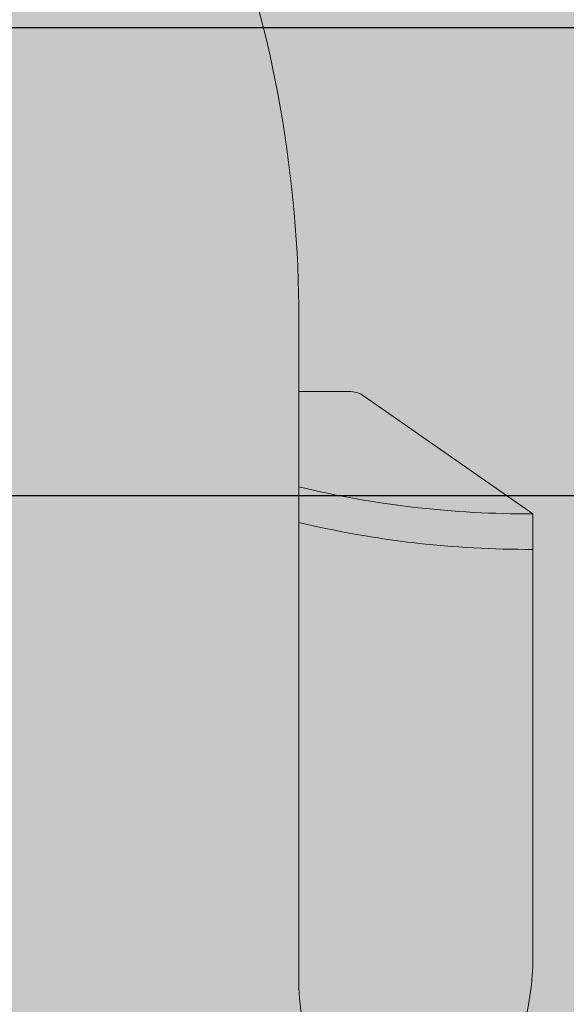
# Model space of a CAD drawing. Units: inches. Extents: x 389 to 971, y 148 to 870.
# Tile 2 of 14: x 515 to 529, y 364 to 389. Entities that reach past the tile are written whole.
import ezdxf

# ---------------------------------------------------------------- set-up
doc = ezdxf.new("R2010")
doc.units = ezdxf.units.IN
doc.header["$MEASUREMENT"] = 0
for name, color, linetype, lineweight in [('A-ANNO-DIMS', 2, 'Continuous', 18), ('C-VEHI', 8, 'Continuous', 13), ('L-GRND-BASE-PATT', 8, 'Continuous', 13)]:
    doc.layers.add(name, color=color, linetype=linetype, lineweight=lineweight)
doc.layers.add('C-VEHI-PATT', color=18, linetype='Continuous', lineweight=13, true_color=0x000000)
doc.layers.add('L-GRND-PATT', color=39, linetype='Continuous', lineweight=13, true_color=0x603913)
doc.styles.get("Standard").update_dxf_attribs({"font": 'arial.ttf'})
doc.dimstyles.get("Standard").update_dxf_attribs({"dimtxt": 8, "dimasz": 8, "dimexe": 0.18, "dimexo": 0.0625, "dimgap": 0.09, "dimtad": 0, "dimtih": 1, "dimtoh": 1, "dimdec": 0, "dimzin": 0, "dimdsep": 46, "dimlunit": 3, "dimtxsty": 'Standard', "dimcen": 0.09, "dimadec": 0, "dimazin": 0, "dimtfac": 1, "dimtdec": 0, "dimtofl": 0, "dimtmove": 0, "dimatfit": 3, "dimfxl": 1, "dimtolj": 1, "dimtzin": 0, "dimarcsym": 0})

# ---------------------------------------------------------------- blocks, each defined once
blk = doc.blocks.new('*U7')
for p, q in [((32.26591480791686, 11.62530558863241), (36.12873726252356, 17.16961494239206)), ((36.12873726252356, 17.16961494239206), (50.93891189819171, 17.16961494239206)), ((32.12291633764599, 9.505833383620029), (32.12291633764599, 11.15369945057711)), ((29.77279020470884, 9.505833383620029), (51.68362801571248, 9.505833383620029))]:
    blk.add_line(p, q)
for centre, major_axis, ratio, start_param, end_param in [((13.03653510440275, 17.00972444508943), (1.2303e-12, 27.41599049210566), 0.8423038695439277, 4.435146050259648, 4.718221029521873), ((14.20086229321332, 17.00972444508943), (1.2303e-12, 27.41599049210566), 0.8423038695439277, 4.435146050259648, 4.718221029521873), ((50.7902773840875, 13.33772416300607), (6.340077547122382, -0.356608581037027), 0.6038335755719145, -1.39555193967809, 1.581314658479915), ((32.74615637525823, 11.15369945057713), (1.313e-13, 0.7399230374541176), 0.8423038695439091, 0.8797135699495516, 1.570796326795045), ((29.77279020470884, -46.66302566589627), (5.12e-14, 56.16885904951626), 0.842303869543976, 7e-16, 0.5903187773915901)]:
    blk.add_ellipse(centre, major_axis=major_axis, ratio=ratio, start_param=start_param, end_param=end_param)
blk = doc.blocks.new('*D53')
at = {"layer": 'A-ANNO-DIMS', "color": 0, "lineweight": -2, "transparency": 16777216}
for p, q in [((397.8910240000004, 396.9189020000002), (397.8910240000004, 404.9189020000001)), ((690.1535240000002, 388.9189020000003), (397.7110240000004, 388.9189020000002)), ((690.1535240000002, 376.9189020000001), (397.7110240000005, 376.9189020000001)), ((397.8910240000005, 368.9189020000001), (397.8910240000005, 360.918902))]:
    blk.add_line(p, q, dxfattribs=at)
at = {"layer": 'A-ANNO-DIMS', "color": 0, "transparency": 16777216}
for points in [[(396.5576906666671, 396.9189020000002), (399.2243573333337, 396.9189020000002), (397.8910240000004, 388.9189020000002)], [(396.5576906666671, 368.9189020000001), (399.2243573333338, 368.9189020000001), (397.8910240000005, 376.9189020000001)]]:
    blk.add_solid(points, dxfattribs=at)
at = {"layer": 'Defpoints', "color": 0, "transparency": 16777216}
for p in [(397.8910240000004, 388.9189020000002), (690.2160240000001, 388.9189020000003), (690.2160240000001, 376.9189020000001)]:
    blk.add_point(p, dxfattribs=at)
at = {"layer": 'A-ANNO-DIMS', "color": 0, "transparency": 16777216, "insert": (397.8910240000004, 382.9189019999999), "char_height": 8, "attachment_point": 5}
blk.add_mtext('\\A1;12', dxfattribs=at)

msp = doc.modelspace()

# ---------------------------------------------------------------- hatches: boundary and pattern name
at = {"layer": 'C-VEHI-PATT'}
h = msp.add_hatch(color=256, dxfattribs=at)
h.dxf.hatch_style = 1
edge = h.paths.add_edge_path()
edge.add_ellipse((550.9021553826709, 381.4331108862803), major_axis=(-43.99405423656321, 1.9369e-12), ratio=0.8423038695439613, start_angle=-29.43856959797762, end_angle=1.8189894035458565e-12, ccw=False)
edge.add_line((514.3535105156315, 402.059641051582), (514.3535105156315, 404.7525403567118))
edge.add_ellipse((514.3535105156316, 404.2643898676136), major_axis=(0.5795420236673633, 2e-16), ratio=0.8423038695437671, start_angle=90.00000000001334, end_angle=127.9331304598466)
edge.add_line((514.0354569934393, 404.6724605914631), (509.5535496243029, 402.1940957519602))
edge.add_ellipse((473.3138688667988, 564.9222417143382), major_axis=(196.5636751472093, 8.4793e-12), ratio=0.8423038695439335, start_angle=-80.7434339928015, end_angle=-77.44506735586577, ccw=False)
edge.add_ellipse((535.9119176052684, 201.7546502845751), major_axis=(239.1273775699096, 1.008988e-10), ratio=0.842303869543627, start_angle=100.2095389971183, end_angle=102.4446272934191)
edge.add_ellipse((979.5722266908713, 375.4013592680145), major_axis=(-488.2195497741742, 7.7268e-12), ratio=0.842303869543895, start_angle=-2.863714607837472, end_angle=2.198540565955285)
edge.add_ellipse((510.1338164488812, 299.4839331720496), major_axis=(70.3178640738586, 3.814e-12), ratio=0.8423038695439212, start_angle=94.08241069114638, end_angle=107.71995322274631, ccw=False)
edge.add_line((505.914122382133, 358.6062023341113), (522.79289864913, 358.606202334111))
edge.add_ellipse((518.5732045823792, 299.4839331720493), major_axis=(-70.31786407385354, 1.4408e-12), ratio=0.8423038695439844, start_angle=252.2800467772501, end_angle=265.91758930884987, ccw=False)
edge.add_ellipse((49.13479434038987, 375.4013592680261), major_axis=(-488.2195497741754, 2.5232e-12), ratio=0.8423038695439587, start_angle=177.8014594340444, end_angle=182.8637146078372)
edge.add_ellipse((492.795103425985, 201.7546502845724), major_axis=(239.12737756976, 4.82267e-11), ratio=0.8423038695441539, start_angle=77.5553727065425, end_angle=79.79046100284327)
edge.add_ellipse((555.3931521644682, 564.9222417143374), major_axis=(-196.5636751472384, 3.62381e-11), ratio=0.8423038695438114, start_angle=77.4450673558726, end_angle=80.74343399280832, ccw=False)
edge.add_line((519.1534714069603, 402.19409575196), (514.671564037824, 404.6724605914631))
edge.add_ellipse((514.3535105156316, 404.2643898676136), major_axis=(0.5795420236673633, 2e-16), ratio=0.8423038695437671, start_angle=52.06686954015338, end_angle=90.00000000001334)
edge.add_line((514.3535105156315, 404.7525403567118), (514.3535105156315, 402.0596410515821))
edge.add_ellipse((477.8048656485917, 381.4331108862812), major_axis=(-43.99405423656326, 6.67e-13), ratio=0.8423038695439753, start_angle=180.0000000000002, end_angle=209.4385695979796, ccw=False)
edge.add_line((521.7989198851549, 381.4331108862806), (521.7989198851549, 379.5923831537828))
edge.add_line((521.7989198851549, 379.5923831537828), (523.2258361412675, 379.5923831537828))
edge.add_ellipse((523.0896049791924, 379.1042326646847), major_axis=(0.5795420236669786, 3.601e-13), ratio=0.8423038695443263, start_angle=45.519789117397124, end_angle=89.99999999996442, ccw=False)
edge.add_line((523.4589887688404, 379.4803801228631), (527.8015488731598, 376.4548385069232))
edge.add_line((527.8015488731598, 376.4548385069232), (527.8015488731597, 364.8548231745798))
edge.add_ellipse((524.8002343791572, 364.9712406163019), major_axis=(0.279312372030448, 4.96584264291768), ratio=0.6038335755719146, start_angle=106.34259195429831, end_angle=270.9979857249735, ccw=False)
edge.add_line((521.7989198851548, 364.2715269884119), (521.7989198851549, 381.4331108862806))
edge.add_ellipse((477.8048656485917, 381.4331108862812), major_axis=(-43.99405423656326, 6.67e-13), ratio=0.8423038695439753, start_angle=180.0000000000001, end_angle=209.4385695979795)
edge.add_ellipse((550.9021553826709, 381.4331108862803), major_axis=(-43.99405423656321, 1.9369e-12), ratio=0.8423038695439613, start_angle=-29.43856959797755, end_angle=1.8539e-12)
edge.add_line((506.9081011461076, 381.43311088628), (506.9081011461074, 364.2715269884121))
edge.add_ellipse((503.9067866521049, 364.9712406163021), major_axis=(-0.2793123720310282, 4.965842642917721), ratio=0.6038335755718928, start_angle=89.00201427501901, end_angle=253.6574080456941, ccw=False)
edge.add_line((500.9054721581025, 364.8548231745812), (500.9054721581025, 376.4548385069235))
edge.add_line((500.9054721581025, 376.4548385069235), (505.3530060491612, 379.5535172937331))
edge.add_ellipse((505.61741605207, 379.1042326646849), major_axis=(-0.5795420236672051, 1.236e-13), ratio=0.842303869543997, start_angle=-89.99999999998778, end_angle=-45.51978911742469, ccw=False)
edge.add_line((505.61741605207, 379.5923831537831), (506.9081011461076, 379.5923831537831))
edge.add_line((506.9081011461076, 379.5923831537831), (506.9081011461076, 381.43311088628))
h = msp.add_hatch(color=256, dxfattribs=at)
h.dxf.hatch_style = 1
edge = h.paths.add_edge_path()
edge.add_ellipse((492.795103425985, 201.7546502845724), major_axis=(239.12737756976, 4.82267e-11), ratio=0.8423038695441539, start_angle=77.5553727065425, end_angle=79.79046100284327)
edge.add_ellipse((555.3931521644682, 564.9222417143374), major_axis=(-196.5636751472384, 3.62381e-11), ratio=0.8423038695438114, start_angle=77.4450673558726, end_angle=80.74343399280832, ccw=False)
edge.add_line((519.1534714069603, 402.19409575196), (519.1534714069603, 394.0892586662818))
edge.add_ellipse((477.8048656485917, 381.4331108862812), major_axis=(-43.99405423656326, 6.67e-13), ratio=0.8423038695439753, start_angle=180.0000000000002, end_angle=197.0185128172791, ccw=False)
edge.add_line((521.7989198851549, 381.4331108862806), (521.7989198851549, 379.5923831537828))
edge.add_line((521.7989198851549, 379.5923831537828), (523.1794038652976, 379.5923831537828))
edge.add_ellipse((523.0896049791924, 379.1042326646847), major_axis=(0.5795420236669786, 3.601e-13), ratio=0.8423038695443263, start_angle=45.519789117397124, end_angle=89.99999999996442, ccw=False)
edge.add_line((523.4589887688405, 379.480380122863), (527.8015488731598, 376.4548385069232))
edge.add_line((527.8015488731598, 376.4548385069232), (527.8015488731597, 364.8548231745798))
edge.add_ellipse((524.8002343791572, 364.9712406163019), major_axis=(0.279312372030448, 4.96584264291768), ratio=0.6038335755719146, start_angle=106.34259195429831, end_angle=270.9979857249735, ccw=False)
edge.add_line((521.7989198851548, 364.2715269884119), (521.7989198851549, 381.4331108862806))
edge.add_ellipse((477.8048656485917, 381.4331108862812), major_axis=(-43.99405423656326, 6.67e-13), ratio=0.8423038695439753, start_angle=180.0000000000001, end_angle=197.018512817279)
edge.add_line((519.1534714069603, 394.0892586662818), (519.1534714069603, 358.6062023341111))
edge.add_line((519.1534714069603, 358.6062023341111), (522.79289864913, 358.606202334111))
edge.add_ellipse((518.5732045823792, 299.4839331720493), major_axis=(-70.31786407385354, 1.4408e-12), ratio=0.8423038695439844, start_angle=252.2800467772501, end_angle=265.91758930884987, ccw=False)
edge.add_ellipse((49.13479434038987, 375.4013592680261), major_axis=(-488.2195497741754, 2.5232e-12), ratio=0.8423038695439587, start_angle=177.8014594340444, end_angle=182.8637146078372)
h = msp.add_hatch(color=256, dxfattribs=at)
h.dxf.hatch_style = 1
edge = h.paths.add_edge_path(flags=16)
edge.add_ellipse((3386.011413077446, 329.726312794031), major_axis=(-2896.629999631248, 1.069454e-10), ratio=0.8423038695494893, start_angle=-0.1208973690315247, end_angle=0.3640763488915013, ccw=False)
edge.add_line((489.3905023836935, 335.8383575186984), (486.2179253655185, 346.1978202249628))
edge.add_ellipse((8782.002602781096, 354.247254279773), major_axis=(-8295.790181758603, 9.87839e-10), ratio=0.8423038695486498, start_angle=0.0555943135052214, end_angle=0.3777641939157137)
edge.add_line((486.4665645878948, 299.5520931219791), (489.4638383140943, 311.3204429697198))
edge = h.paths.add_edge_path(flags=16)
edge.add_ellipse((512.1608573463288, 287.5825181681774), major_axis=(62.33048198263887, 2.0798e-12), ratio=0.8423038695439498, start_angle=94.8700695971331, end_angle=112.791914877584)
edge.add_line((491.3642517254777, 337.0752369161335), (489.6529508739416, 349.9015767089268))
edge.add_ellipse((510.1338164488795, 298.7862183048575), major_axis=(64.04807894948699, 3.9006e-12), ratio=0.8423038695439252, start_angle=94.27742096304979, end_angle=111.83495379670401, ccw=False)
edge.add_line((506.1068129054811, 352.6274231954524), (522.600208125781, 352.6274231954521))
edge.add_ellipse((518.5732045823798, 298.7862183048586), major_axis=(64.04807894948067, 3.24e-14), ratio=0.8423038695439885, start_angle=68.16504620328948, end_angle=85.72257903694378, ccw=False)
edge.add_line((539.05407015732, 349.9015767089259), (537.3427693057835, 337.0752369161327))
edge.add_ellipse((516.5461636849332, 287.5825181681899), major_axis=(62.33048198262021, 1.5954e-12), ratio=0.8423038695439995, start_angle=67.20808512240782, end_angle=85.12993040286212)
edge.add_line((521.0080028322477, 339.9490379899644), (507.6990181990146, 339.9490379899646))
edge = h.paths.add_edge_path(flags=16)
edge.add_ellipse((514.3535105156315, 391.3730654902235), major_axis=(-115.1512533244504, 1.8736e-12), ratio=0.8423038695439684, start_angle=76.4018653097696, end_angle=103.5981346902308)
edge.add_line((537.3427693057832, 296.3333211885938), (537.342769305783, 281.5897392316151))
edge.add_ellipse((514.3535105156313, 376.6294835332447), major_axis=(-115.1512533244486, 9.02e-13), ratio=0.8423038695439828, start_angle=76.40186530976922, end_angle=103.59813469023032, ccw=False)
edge.add_line((491.3642517254773, 281.5897392316156), (491.3642517254774, 296.3333211885945))
edge = h.paths.add_edge_path()
edge.add_ellipse((8782.002602781105, 354.2472542798386), major_axis=(-8296.949265805946, 5.39345e-11), ratio=0.8423038695428886, start_angle=0.3838667787920247, end_angle=0.5282714718170651)
edge.add_ellipse((8782.002602781105, 354.2472542798386), major_axis=(-8296.949265805946, 5.39345e-11), ratio=0.8423038695428886, start_angle=0.5282714718170651, end_angle=0.6465540970606384)
edge.add_ellipse((488.1158467995968, 260.6509346628684), major_axis=(2.318168094668909, 7.48e-14), ratio=0.8423038695439647, start_angle=180.6465540970884, end_angle=269.9999999999081)
edge.add_line((488.115846799593, 258.6983327064755), (491.3642517254771, 258.6983327064753))
edge.add_line((491.3642517254771, 258.6983327064753), (491.3642517254771, 274.201106836649))
edge.add_ellipse((493.6824198201462, 273.9438556676354), major_axis=(-2.318168094668919, 1.896e-13), ratio=0.8423038695439611, start_angle=-89.99999999999523, end_angle=4.718003765447065e-12, ccw=False)
edge.add_line((493.6824198201462, 275.8964576240284), (535.3300149439905, 275.8964576240277))
edge.add_ellipse((535.024601211114, 273.9438556676347), major_axis=(2.318168094668976, 2.946e-13), ratio=0.8423038695439647, start_angle=-7.275957614183426e-12, end_angle=89.99999999998943, ccw=False)
edge.add_line((537.342769305783, 273.9438556676347), (537.3427693057827, 258.698332706474))
edge.add_line((537.3427693057827, 258.698332706474), (540.591174231666, 258.6983327064739))
edge.add_ellipse((540.5911742316634, 260.6509346628669), major_axis=(-2.318168094668839, 2.143e-13), ratio=0.8423038695440144, start_angle=90.00000000008203, end_angle=179.3534459029346)
edge.add_ellipse((-7753.295581726658, 354.2472542799028), major_axis=(-8296.949265782761, 2.068448e-10), ratio=0.8423038695442414, start_angle=179.3534459029388, end_angle=179.3813568036815)
edge.add_ellipse((-7753.295581726658, 354.2472542799028), major_axis=(-8296.949265782761, 2.068448e-10), ratio=0.8423038695442414, start_angle=179.3813568036815, end_angle=179.4717285281828)
edge.add_ellipse((-7753.295581726658, 354.2472542799028), major_axis=(-8296.949265782761, 2.068448e-10), ratio=0.8423038695442414, start_angle=179.4717285281828, end_angle=179.6161332212082)
edge.add_ellipse((-7753.295581726658, 354.2472542799028), major_axis=(-8296.949265782761, 2.068448e-10), ratio=0.8423038695442414, start_angle=179.6161332212082, end_angle=180.090229088595)
edge.add_ellipse((-7753.295581726658, 354.2472542799028), major_axis=(-8296.949265782761, 2.068448e-10), ratio=0.8423038695442414, start_angle=180.090229088595, end_angle=180.134986576859)
edge.add_ellipse((129.8867725257751, 372.4897205359271), major_axis=(-413.7373561031673, 2.44623e-11), ratio=0.8423038695441432, start_angle=180.1806905311865, end_angle=182.1799503136479)
edge.add_ellipse((129.8867725257751, 372.4897205359271), major_axis=(-413.7373561031673, 2.44623e-11), ratio=0.8423038695441432, start_angle=182.1799503136479, end_angle=183.6504275857017)
edge.add_ellipse((492.7951034259847, 196.3854951855023), major_axis=(245.3971626940514, 1.422861e-10), ratio=0.8423038695444116, start_angle=76.21947101046817, end_angle=77.87403444768196)
edge.add_ellipse((49.13479434038987, 375.4013592680261), major_axis=(-488.2195497741754, 2.5232e-12), ratio=0.8423038695439587, start_angle=177.8014594340445, end_angle=182.8637146078372, ccw=False)
edge.add_ellipse((518.5732045823792, 299.4839331720493), major_axis=(-70.31786407385354, 1.4408e-12), ratio=0.8423038695439844, start_angle=252.2800467772501, end_angle=265.9175893088498)
edge.add_line((522.79289864913, 358.606202334111), (505.9141223821329, 358.6062023341113))
edge.add_ellipse((510.1338164488812, 299.4839331720496), major_axis=(70.3178640738586, 3.814e-12), ratio=0.8423038695439212, start_angle=94.08241069114636, end_angle=107.7199532227462)
edge.add_ellipse((979.5722266908713, 375.4013592680145), major_axis=(-488.2195497741742, 7.7268e-12), ratio=0.842303869543895, start_angle=-2.863714607837494, end_angle=2.198540565955284, ccw=False)
edge.add_ellipse((535.9119176052733, 196.3854951855018), major_axis=(-245.3971626940985, 1.013648e-10), ratio=0.8423038695442548, start_angle=-77.87403444769295, end_angle=-76.2194710104792)
edge.add_ellipse((898.8202485054873, 372.489720535918), major_axis=(413.7373561031672, 1.26113e-11), ratio=0.8423038695441164, start_angle=176.3495724142985, end_angle=177.8200496863523)
edge.add_ellipse((898.8202485054873, 372.489720535918), major_axis=(413.7373561031672, 1.26113e-11), ratio=0.8423038695441164, start_angle=177.8200496863523, end_angle=179.8643876095591)
edge.add_ellipse((8782.002602781105, 354.2472542798386), major_axis=(-8296.949265805946, 5.39345e-11), ratio=0.8423038695428886, start_angle=-0.1349865768573029, end_angle=-0.090229088593484)
edge.add_ellipse((8782.002602781105, 354.2472542798386), major_axis=(-8296.949265805946, 5.39345e-11), ratio=0.8423038695428886, start_angle=-0.090229088593484, end_angle=0.3838667787920247)
edge = h.paths.add_edge_path(flags=16)
edge.add_ellipse((-2357.304392046186, 329.7263127941099), major_axis=(2896.629999631251, 5.35614e-11), ratio=0.8423038695445265, start_angle=-0.3640763488920631, end_angle=0.1208973690309369)
edge.add_line((539.3165186475693, 335.8383575187012), (542.4890956657468, 346.1978202249727))
edge.add_ellipse((-7753.295581749842, 354.2472542800017), major_axis=(8295.790181758617, 3.2664368e-09), ratio=0.8423038695525207, start_angle=-0.37776419393310334, end_angle=-0.055594313522590255, ccw=False)
edge.add_line((542.240456443367, 299.5520931219743), (539.2431827171666, 311.3204429697195))
h = msp.add_hatch(color=256, dxfattribs=at)
h.dxf.hatch_style = 1
edge = h.paths.add_edge_path()
edge.add_ellipse((523.0896049791924, 379.1042326646847), major_axis=(0.5795420236669786, 3.601e-13), ratio=0.8423038695443263, start_angle=45.51978911739708, end_angle=89.99999999996442)
edge.add_line((523.0896049791935, 379.5923831537828), (521.7989198851549, 379.5923831537828))
edge.add_line((521.7989198851549, 379.5923831537828), (521.7989198851549, 377.1452135063881))
edge.add_ellipse((527.6763152236028, 394.5417217261543), major_axis=(-21.47347468097256, 2.8383e-12), ratio=0.8423038695438576, start_angle=71.33250450740293, end_angle=90.39670985998444)
edge.add_line((527.8015488731598, 376.4548385069232), (523.4589887688408, 379.4803801228628))
h = msp.add_hatch(color=256, dxfattribs=at)
h.dxf.hatch_style = 1
edge = h.paths.add_edge_path()
edge.add_ellipse((523.0896049791924, 379.1042326646847), major_axis=(0.5795420236669786, 3.601e-13), ratio=0.8423038695443263, start_angle=45.51978911739708, end_angle=89.99999999996442)
edge.add_line((523.0896049791935, 379.5923831537828), (521.7989198851549, 379.5923831537828))
edge.add_line((521.7989198851549, 379.5923831537828), (521.7989198851549, 377.1452135063881))
edge.add_ellipse((527.6763152236028, 394.5417217261543), major_axis=(-21.47347468097256, 2.8383e-12), ratio=0.8423038695438576, start_angle=71.33250450740293, end_angle=90.39670985998444)
edge.add_line((527.8015488731598, 376.4548385069232), (523.4589887688408, 379.4803801228628))
h = msp.add_hatch(color=256, dxfattribs=at)
h.dxf.hatch_style = 1
edge = h.paths.add_edge_path()
edge.add_ellipse((523.0896049791924, 379.1042326646847), major_axis=(0.5795420236669786, 3.601e-13), ratio=0.8423038695443263, start_angle=45.51978911739708, end_angle=89.99999999996442)
edge.add_line((523.0896049791935, 379.5923831537828), (521.7989198851549, 379.5923831537828))
edge.add_line((521.7989198851549, 379.5923831537828), (521.7989198851549, 377.1452135063881))
edge.add_ellipse((527.6763152236028, 394.5417217261543), major_axis=(-21.47347468097256, 2.8383e-12), ratio=0.8423038695438576, start_angle=71.33250450740293, end_angle=90.39670985998444)
edge.add_line((527.8015488731598, 376.4548385069232), (523.4589887688408, 379.4803801228628))
h = msp.add_hatch(color=256, dxfattribs=at)
h.dxf.hatch_style = 1
edge = h.paths.add_edge_path()
edge.add_ellipse((527.6763152236028, 394.5417217261543), major_axis=(-21.47347468097256, 2.8383e-12), ratio=0.8423038695438576, start_angle=71.33250450740297, end_angle=90.39670985998453, ccw=False)
edge.add_line((521.7989198851549, 377.1452135063881), (521.7989198851549, 376.2332584772058))
edge.add_ellipse((527.6763152236027, 393.629766696972), major_axis=(-21.47347468097092, 1.1981e-12), ratio=0.8423038695439196, start_angle=71.33250450739882, end_angle=90.3967098599804)
edge.add_line((527.8015488731598, 375.5428834777409), (527.8015488731598, 376.4548385069232))
h = msp.add_hatch(color=256, dxfattribs=at)
h.dxf.hatch_style = 1
edge = h.paths.add_edge_path()
edge.add_ellipse((527.6763152236027, 393.629766696972), major_axis=(-21.47347468097092, 1.1981e-12), ratio=0.8423038695439196, start_angle=71.33250450739882, end_angle=90.39670985998049, ccw=False)
edge.add_line((521.7989198851549, 376.2332584772058), (521.7989198851548, 364.2715269884119))
edge.add_ellipse((524.8002343791572, 364.9712406163019), major_axis=(0.279312372030448, 4.96584264291768), ratio=0.6038335755719146, start_angle=106.3425919542983, end_angle=270.9979857249735)
edge.add_line((527.8015488731597, 364.8548231745798), (527.8015488731598, 375.5428834777409))
h = msp.add_hatch(color=256, dxfattribs=at)
h.dxf.hatch_style = 1
edge = h.paths.add_edge_path()
edge.add_ellipse((527.6763152236027, 393.629766696972), major_axis=(-21.47347468097092, 1.1981e-12), ratio=0.8423038695439196, start_angle=71.33250450739882, end_angle=90.39670985998049, ccw=False)
edge.add_line((521.7989198851549, 376.2332584772058), (521.7989198851548, 364.2715269884119))
edge.add_ellipse((524.8002343791572, 364.9712406163019), major_axis=(0.279312372030448, 4.96584264291768), ratio=0.6038335755719146, start_angle=106.3425919542983, end_angle=270.9979857249735)
edge.add_line((527.8015488731597, 364.8548231745798), (527.8015488731598, 375.5428834777409))
at = {"layer": 'L-GRND-BASE-PATT'}
h = msp.add_hatch(color=256, dxfattribs=at)
h.dxf.hatch_style = 1
edge = h.paths.add_edge_path(flags=16)
edge.add_ellipse((8782.002602781105, 354.2472542798386), major_axis=(-8296.949265805946, 5.39345e-11), ratio=0.8423038695428886, start_angle=-0.0902290885933894, end_angle=0.3838667787920258, ccw=False)
edge.add_ellipse((485.0533369751568, 368.2895347624687), major_axis=(-1.159084047334488, 1.838e-13), ratio=0.8423038695439892, start_angle=9.094947017729282e-12, end_angle=90.00000000000898, ccw=False)
edge.add_line((483.8942529278224, 368.2895347624687), (483.8942529278225, 387.6039063360424))
edge.add_ellipse((485.0533369751571, 387.2465553762829), major_axis=(1.159084047334488, 1.838e-13), ratio=0.8423038695439892, start_angle=89.99999999999102, end_angle=179.9999999999909, ccw=False)
edge.add_line((485.0533369751572, 388.2228563544795), (485.5047440247956, 388.2228563544795))
edge.add_ellipse((898.8202485054873, 372.489720535918), major_axis=(413.7373561031672, 1.26113e-11), ratio=0.8423038695441164, start_angle=176.3495724142986, end_angle=177.8200496863524, ccw=False)
edge.add_ellipse((535.9119176052733, 196.3854951855018), major_axis=(-245.3971626940985, 1.013648e-10), ratio=0.8423038695442548, start_angle=-77.87403444769302, end_angle=-76.2194710104792, ccw=False)
edge.add_ellipse((535.9119176052684, 201.7546502845751), major_axis=(239.1273775699096, 1.008988e-10), ratio=0.842303869543627, start_angle=100.20953899711827, end_angle=102.44462729341922, ccw=False)
edge.add_ellipse((473.3138688667988, 564.9222417143382), major_axis=(196.5636751472093, 8.4793e-12), ratio=0.8423038695439335, start_angle=-80.74343399280163, end_angle=-77.44506735586587)
edge.add_line((509.5535496243029, 402.1940957519602), (514.3535105156315, 404.8483349684994))
edge.add_line((514.3535105156315, 404.8483349684994), (514.3535105156315, 404.7971763262221))
edge.add_ellipse((514.3535105156316, 404.2643898676136), major_axis=(0.5795420236673633, 2e-16), ratio=0.8423038695437671, start_angle=52.06686954015339, end_angle=90.00000000001342, ccw=False)
edge.add_line((514.671564037824, 404.672460591463), (519.1534714069603, 402.19409575196))
edge.add_ellipse((555.3931521644682, 564.9222417143374), major_axis=(-196.5636751472384, 3.62381e-11), ratio=0.8423038695438114, start_angle=77.44506735587258, end_angle=80.74343399280833)
edge.add_ellipse((492.795103425985, 201.7546502845724), major_axis=(239.12737756976, 4.82267e-11), ratio=0.8423038695441539, start_angle=77.55537270654253, end_angle=79.7904610028433, ccw=False)
edge.add_ellipse((492.7951034259847, 196.3854951855023), major_axis=(245.3971626940514, 1.422861e-10), ratio=0.8423038695444116, start_angle=76.21947101046823, end_angle=77.87403444768199, ccw=False)
edge.add_ellipse((129.8867725257751, 372.4897205359271), major_axis=(-413.7373561031673, 2.44623e-11), ratio=0.8423038695441432, start_angle=182.179950313648, end_angle=183.6504275857018, ccw=False)
edge.add_line((543.2022770064673, 388.2228563544788), (544.0779382625514, 388.2228563544787))
edge.add_ellipse((543.6536840561057, 387.2465553762822), major_axis=(-1.159084047334545, 1.527e-13), ratio=0.8423038695438989, start_angle=180.0000000000075, end_angle=270.00000000000756, ccw=False)
edge.add_line((544.8127681034401, 387.2465553762826), (544.8127681034399, 367.9321838027083))
edge.add_ellipse((543.6536840561054, 368.2895347624679), major_axis=(1.159084047334544, 7.24e-14), ratio=0.8423038695439478, start_angle=269.9999999999964, end_angle=359.9999999999964, ccw=False)
edge.add_ellipse((-7753.295581726658, 354.2472542799028), major_axis=(-8296.949265782761, 2.068448e-10), ratio=0.8423038695442414, start_angle=179.6161332212083, end_angle=180.0902290885951, ccw=False)
edge.add_line((543.3912265319653, 298.6607849184036), (544.0779382625504, 298.6607849184036))
edge.add_ellipse((543.6536840561046, 297.6844839402071), major_axis=(1.159084047334431, 1.769e-13), ratio=0.8423038695439814, start_angle=-1.1482370609883219e-11, end_angle=89.99999999999119, ccw=False)
edge.add_line((544.8127681034391, 297.684483940207), (544.8127681034387, 278.3701123666333))
edge.add_ellipse((543.6536840561043, 278.727463326393), major_axis=(-1.159084047334431, 2.574e-13), ratio=0.8423038695440306, start_angle=90.00000000001268, end_angle=180.0000000000099, ccw=False)
edge.add_line((543.6536840561045, 277.7511623481965), (543.1566278692261, 277.7511623481965))
edge.add_ellipse((-7753.295581726658, 354.2472542799028), major_axis=(-8296.949265782761, 2.068448e-10), ratio=0.8423038695442414, start_angle=179.3813568036816, end_angle=179.4717285281829, ccw=False)
edge.add_ellipse((542.4236240941387, 263.2762864208561), major_axis=(-1.738626071001761, 2.132e-13), ratio=0.8423038695439151, start_angle=179.3717627838137, end_angle=248.464756601011, ccw=False)
edge.add_ellipse((-7753.875123750511, 354.2472542780016), major_axis=(-8298.740341433751, 2.4782644722e-06), ratio=0.8423038662721074, start_angle=179.3534459200609, end_angle=179.3717628008941, ccw=False)
edge.add_ellipse((540.0116322079951, 260.6509346628677), major_axis=(-4.109243751168186, 2.384e-13), ratio=0.842303869543976, start_angle=90.0000000000635, end_angle=179.3534459029233, ccw=False)
edge.add_line((540.0116322079991, 257.1897027503593), (488.6953888232593, 257.1897027503609))
edge.add_ellipse((488.6953888232669, 260.6509346628715), major_axis=(4.10924375117072, 1.262e-13), ratio=0.8423038695439824, start_angle=180.6465540970565, end_angle=269.9999999998589, ccw=False)
edge.add_ellipse((8782.582144816053, 354.2472542821698), major_axis=(-8298.740341477976, 1.8591886369e-06), ratio=0.8423038720186145, start_angle=0.6282372290784792, end_angle=0.6465541099116194, ccw=False)
edge.add_ellipse((486.2833969371199, 263.2762864208594), major_axis=(-1.738626071002378, 2.7e-13), ratio=0.8423038695439394, start_angle=-68.46475649596817, end_angle=0.6282372161796275, ccw=False)
edge.add_ellipse((8782.002602781105, 354.2472542798386), major_axis=(-8296.949265805946, 5.39345e-11), ratio=0.8423038695428886, start_angle=0.5282714718171064, end_angle=0.6465540970606867, ccw=False)
edge.add_line((485.5503931620382, 277.7511623481972), (484.6290827687102, 277.7511623481972))
edge.add_ellipse((485.0533369751559, 278.7274633263938), major_axis=(-1.159084047334545, 3.11e-13), ratio=0.8423038695439968, start_angle=1.5404566511278972e-11, end_angle=90.000000000012, ccw=False)
edge.add_line((483.8942529278214, 278.7274633263938), (483.8942529278216, 298.0418348999672))
edge.add_ellipse((485.053336975156, 297.6844839402078), major_axis=(1.159084047334488, 1.025e-13), ratio=0.8423038695440382, start_angle=89.99999999999488, end_angle=179.9999999999949, ccw=False)
edge = h.paths.add_edge_path(flags=0)
edge.add_ellipse((8782.002602781096, 354.247254279773), major_axis=(-8295.790181758603, 9.87839e-10), ratio=0.8423038695486498, start_angle=0.05559431350519617, end_angle=0.37776419391582294, ccw=False)
edge.add_line((486.2179253655185, 346.1978202249628), (489.3905023836935, 335.8383575186984))
edge.add_ellipse((3386.011413077446, 329.726312794031), major_axis=(-2896.629999631248, 1.069454e-10), ratio=0.8423038695494893, start_angle=-0.1208973690315206, end_angle=0.3640763488915184)
edge.add_line((489.4638383140943, 311.3204429697198), (486.4665645878948, 299.5520931219791))
edge = h.paths.add_edge_path(flags=0)
edge.add_ellipse((514.3535105156315, 391.3730654902235), major_axis=(-115.1512533244504, 1.8736e-12), ratio=0.8423038695439684, start_angle=76.4018653097696, end_angle=103.5981346902308)
edge.add_line((537.3427693057832, 296.3333211885938), (537.342769305783, 281.5897392316151))
edge.add_ellipse((514.3535105156313, 376.6294835332447), major_axis=(-115.1512533244486, 9.02e-13), ratio=0.8423038695439828, start_angle=76.40186530976922, end_angle=103.59813469023032, ccw=False)
edge.add_line((491.3642517254773, 281.5897392316156), (491.3642517254774, 296.3333211885945))
edge = h.paths.add_edge_path(flags=0)
edge.add_line((491.3642517254777, 337.0752369161334), (489.6529508739416, 349.9015767089268))
edge.add_ellipse((510.1338164488795, 298.7862183048575), major_axis=(64.04807894948699, 3.9006e-12), ratio=0.8423038695439252, start_angle=94.27742096304979, end_angle=111.83495379670401, ccw=False)
edge.add_line((506.106812905481, 352.6274231954524), (522.600208125781, 352.6274231954521))
edge.add_ellipse((518.5732045823798, 298.7862183048586), major_axis=(64.04807894948067, 3.24e-14), ratio=0.8423038695439885, start_angle=68.16504620328948, end_angle=85.72257903694378, ccw=False)
edge.add_line((539.05407015732, 349.9015767089259), (537.3427693057835, 337.0752369161327))
edge.add_ellipse((516.5461636849332, 287.5825181681899), major_axis=(62.33048198262021, 1.5954e-12), ratio=0.8423038695439995, start_angle=67.20808512240782, end_angle=85.12993040286212)
edge.add_line((521.0080028322477, 339.9490379899644), (507.6990181990146, 339.9490379899646))
edge.add_ellipse((512.1608573463288, 287.5825181681774), major_axis=(62.33048198263887, 2.0798e-12), ratio=0.8423038695439498, start_angle=94.8700695971331, end_angle=112.791914877584)
edge = h.paths.add_edge_path(flags=0)
edge.add_ellipse((493.6824198201462, 273.9438556676354), major_axis=(-2.318168094668919, 1.896e-13), ratio=0.8423038695439611, start_angle=-89.99999999999523, end_angle=4.718003765447065e-12, ccw=False)
edge.add_line((493.6824198201462, 275.8964576240284), (535.3743409680425, 275.8964576240277))
edge.add_ellipse((535.024601211114, 273.9438556676347), major_axis=(2.318168094668976, 2.946e-13), ratio=0.8423038695439647, start_angle=-7.275957614183426e-12, end_angle=89.99999999998943, ccw=False)
edge.add_line((537.342769305783, 273.9438556676347), (537.3427693057827, 258.698332706474))
edge.add_line((537.3427693057827, 258.698332706474), (540.5911742316662, 258.6983327064739))
edge.add_ellipse((540.5911742316634, 260.6509346628669), major_axis=(-2.318168094668839, 2.143e-13), ratio=0.8423038695440144, start_angle=90.00000000008203, end_angle=179.3534459029346)
edge.add_line((540.5911742316662, 258.6983327064739), (487.7691399811528, 258.6983327064755))
edge.add_ellipse((488.1158467995968, 260.6509346628684), major_axis=(2.318168094668909, 7.48e-14), ratio=0.8423038695439647, start_angle=180.6465540970884, end_angle=269.9999999999081)
edge.add_line((488.1158467995931, 258.6983327064755), (491.3642517254771, 258.6983327064754))
edge.add_line((491.3642517254771, 258.6983327064754), (491.3642517254771, 274.2384428182294))
h.paths.add_polyline_path([(746.1375687288224, 327.3223047166553), (750.1400147212453, 327.3223047166553), (750.1400147212453, 326.2830696147227), (798.1693712998389, 326.2830696147227), (798.1693712998389, 327.3223047166553), (802.1718172922616, 327.3223047166553), (802.1718172922616, 309.9783792024682, -0.1904762075443491), (746.1375687288224, 309.9783668090107)], flags=16)
h.paths.add_polyline_path([(782.1595875801748, 313.5684994305933), (782.1595893317732, 309.0414930416419, -0.0496282101666581), (766.1497986905329, 309.0414910503953), (766.1498004421323, 313.5684994305933)], flags=0)
h.paths.add_polyline_path([(755.1858908233534, 344.9352232902417), (755.1858908233534, 373.916311072083), (788.1243995226009, 373.916311072083), (788.1243995226009, 344.9352232902417)], flags=16)
h.paths.add_polyline_path([(757.1858908233535, 346.9352232902417), (757.1858908233535, 371.916311072083), (786.1243995226009, 371.916311072083), (786.1243995226009, 346.9352232902417)], flags=0)
h.paths.add_polyline_path([(803.6445810111745, 338.4878931208803), (803.6445810111745, 342.4903391133031), (804.6838161131072, 342.4903391133031), (804.6838161131072, 390.5196956918968), (803.6445810111748, 390.5196956918968), (803.6445810111748, 394.5221416843196), (820.9885065253617, 394.5221416843196, -0.1904762075443491), (820.9885189188192, 338.4878931208803)], flags=16)
h.paths.add_polyline_path([(806.8706930931005, 326.6963103558256), (806.4254411777042, 327.1415622712219), (806.4723791864895, 326.6297175483474)], flags=16)
h.paths.add_polyline_path([(822.0328146004263, 317.4007976138144), (822.1941503181826, 317.8932883068639), (821.562628166435, 317.9885306563034)], flags=16)
h.paths.add_polyline_path([(817.3983862972365, 358.5001248341902), (817.3983862972365, 374.5099119722327), (821.9253926861879, 374.5099137238312, -0.049628210166658), (821.9253946774346, 358.5001230825909)], flags=0)
h.paths.add_polyline_path([(808.1446344648577, 418.9736619306146), (808.2246858861593, 418.5632188717996), (808.5395491501399, 418.5787472453325)], flags=16)
h.paths.add_polyline_path([(820.3158762739024, 412.6690288868844), (820.4772119916585, 413.161519579934), (819.8456898399113, 413.2567619293735)], flags=16)
h.paths.add_polyline_path([(466.3155093563569, 235.5246322146605), (517.3806533266912, 235.5246322146605), (517.3806533266912, 244.4269231682286), (466.3155093563569, 244.4269231682286)], flags=24)
h.paths.add_polyline_path([(739.8737195480014, 256.2000079819968), (815.4040239338423, 256.2000079819968), (815.4040239338423, 265.3453807094367), (739.8737195480014, 265.3453807094367)], flags=24)
h.paths.add_polyline_path([(750.6081538187397, 393.6666679930368), (791.5680640722773, 393.6666679930368), (791.5680640722773, 412.3933175868746), (750.6081538187397, 412.3933175868746)], flags=24)
h.paths.add_polyline_path([(438.9630812812552, 410.0618566955462), (484.6203810968238, 410.0618566955462), (484.6203810968238, 429.1217352891893), (438.9630812812552, 429.1217352891893)], flags=24)
edge = h.paths.add_edge_path()
edge.add_line((839.2160244416713, 285.6445131961097), (611.8786784019748, 285.6445131961099))
edge.add_line((611.8786784019748, 285.6445131961099), (604.3870116090119, 285.6445131961097))
edge.add_line((604.3870116090119, 285.6445131961097), (595.3870116090119, 285.6445131961097))
edge.add_line((595.3870116090119, 285.6445131961097), (595.3870116090118, 370.1553848722774))
edge.add_line((595.3870116090118, 370.1553848722774), (604.0816928471932, 370.1553848722774))
edge.add_line((604.0816928471932, 370.1553848722774), (604.0816928471932, 371.3788335667469))
edge.add_line((604.0816928471932, 371.3788335667469), (632.0194586761203, 371.3788335667469))
edge.add_arc((604.0816928471932, 370.1553848722773), 27.96454158787471, 2.507490703587644, 90.00000000000003)
edge.add_line((604.0816928471932, 398.1199264601519), (599.8870116090108, 398.1652144688576))
edge.add_line((599.8870116090108, 398.1652144688576), (604.4225424425357, 398.1652144688576))
edge.add_arc((604.4225424425357, 428.4020866923496), 30.23687222349201, 270.0000000000002, 357.492509296413)
edge.add_line((634.6304631740308, 427.0792235325719), (604.4225424425357, 427.0792235325719))
edge.add_line((604.4225424425357, 427.0792235325719), (604.4225424425357, 428.4020866923497))
edge.add_line((604.4225424425357, 428.4020866923497), (599.8870116090119, 428.4020866923497))
edge.add_line((599.8870116090119, 428.4020866923497), (595.3870116090116, 428.4020866923497))
edge.add_line((595.3870116090116, 428.4020866923497), (595.3870116090118, 434.6445131961097))
edge.add_line((595.3870116090118, 434.6445131961097), (585.0790669792458, 434.6445131961097))
edge.add_line((585.0790669792458, 434.6445131961097), (540.3921730610418, 434.6445131961097))
edge.add_line((540.3921730610418, 434.6445131961097), (526.712508448134, 434.6445131961097))
edge.add_line((526.712508448134, 434.6445131961097), (488.4094553949635, 434.6445131961097))
edge.add_line((488.4094553949635, 434.6445131961097), (432.2160244416713, 434.6445131961097))
edge.add_line((432.2160244416713, 434.6445131961097), (432.2160244416713, 243.6445131961098))
edge.add_line((432.2160244416713, 243.6445131961098), (437.2160244416714, 243.6445131961098))
edge.add_line((437.2160244416714, 243.6445131961098), (437.2160244416714, 234.6445131961098))
edge.add_line((437.2160244416714, 234.6445131961098), (581.2160244416713, 234.6445131961098))
edge.add_line((581.2160244416713, 234.6445131961098), (581.2160244416713, 238.6445131961097))
edge.add_line((581.2160244416713, 238.6445131961097), (581.2160244416713, 243.6445131961098))
edge.add_line((581.2160244416713, 243.6445131961098), (590.2160244416713, 243.6445131961098))
edge.add_line((590.2160244416713, 243.6445131961098), (590.2160244416713, 238.6445131961097))
edge.add_line((590.2160244416713, 238.6445131961097), (839.2160244416713, 238.6445131961098))
edge.add_line((839.2160244416713, 238.6445131961098), (839.2160244416713, 285.6445131961097))
at = {"layer": 'L-GRND-PATT'}
h = msp.add_hatch(dxfattribs=at)
h.set_pattern_fill('EARTH', color=256, angle=45)
h.set_pattern_definition([(45, (0, 0), (0, 8.980256121069154), [6.349999999999999, -6.349999999999999]), (45, (-1.683798022700466, 1.683798022700466), (0, 8.980256121069154), [6.349999999999999, -6.349999999999999]), (45, (-3.367596045400933, 3.367596045400933), (0, 8.980256121069154), [6.349999999999999, -6.349999999999999]), (135, (-3.367596045400933, 4.490128060534576), (-8.980256121069154, 0), [6.349999999999999, -6.349999999999999]), (135, (-1.683798022700466, 6.173926083235043), (-8.980256121069154, 0), [6.349999999999999, -6.349999999999999]), (135, (0, 7.85772410593551), (-8.980256121069154, 0), [6.349999999999999, -6.349999999999999])])
h.paths.add_polyline_path([(432.2160244416713, 243.6445131961098), (437.2160244416714, 243.6445131961098), (437.2160244416714, 234.6445131961098), (581.2160244416713, 234.6445131961098), (581.2160244416713, 238.6445131961097), (581.2160244416713, 243.6445131961098), (590.2160244416713, 243.6445131961098), (590.2160244416713, 238.6445131961097), (839.2160244416713, 238.6445131961098), (839.2160244416712, 285.6445131961097), (810.0513609197296, 285.6445131961097), (733.8056934525983, 285.6445131961099), (684.2433676403508, 285.6445131961098), (611.8786784019748, 285.6445131961099), (604.3870116090119, 285.6445131961097), (595.3870116090119, 285.6445131961097), (595.3870116090118, 370.1553848722774), (604.0816928471932, 370.1553848722774), (604.0816928471932, 371.3788335667469), (632.0194586761203, 371.3788335667469, 0.4014527144963568), (604.0816928471932, 398.119926460152), (599.8870116090127, 398.1652144688576), (604.4225424425357, 398.1652144688576, 0.4014527144963579), (634.6304631740308, 427.0792235325719), (604.4225424425357, 427.0792235325719), (604.4225424425357, 428.4020866923497), (599.8870116090119, 428.4020866923497), (595.3870116090116, 428.4020866923497), (595.3870116090118, 434.6445131961097), (585.0790669792458, 434.6445131961097), (540.3921730610418, 434.6445131961097), (526.712508448134, 434.6445131961097), (488.4094553949635, 434.6445131961097), (432.2160244416713, 434.6445131961097)])
edge = h.paths.add_edge_path(flags=16)
edge.add_line((483.8942529278214, 278.7274633263938), (483.8942529278216, 298.2563878122772))
edge.add_ellipse((485.053336975156, 297.6844839402078), major_axis=(1.159084047334488, 1.025e-13), ratio=0.8423038695440382, start_angle=89.99999999999488, end_angle=179.9999999999949, ccw=False)
edge.add_ellipse((8782.002602781105, 354.2472542798386), major_axis=(-8296.949265805946, 5.39345e-11), ratio=0.8423038695428886, start_angle=-0.0902290885933894, end_angle=0.3838667787920258, ccw=False)
edge.add_ellipse((485.0533369751568, 368.2895347624687), major_axis=(-1.159084047334488, 1.838e-13), ratio=0.8423038695439892, start_angle=9.094947017729282e-12, end_angle=90.00000000000898, ccw=False)
edge.add_line((483.8942529278224, 368.2895347624687), (483.8942529278225, 387.8184592483523))
edge.add_ellipse((485.0533369751571, 387.2465553762829), major_axis=(1.159084047334488, 1.838e-13), ratio=0.8423038695439892, start_angle=89.99999999999102, end_angle=179.9999999999909, ccw=False)
edge.add_ellipse((898.8202485054873, 372.489720535918), major_axis=(413.7373561031672, 1.26113e-11), ratio=0.8423038695441164, start_angle=176.3495724142986, end_angle=177.8200496863524, ccw=False)
edge.add_ellipse((535.9119176052733, 196.3854951855018), major_axis=(-245.3971626940985, 1.013648e-10), ratio=0.8423038695442548, start_angle=-77.87403444769302, end_angle=-76.2194710104792, ccw=False)
edge.add_ellipse((535.9119176052684, 201.7546502845751), major_axis=(239.1273775699096, 1.008988e-10), ratio=0.842303869543627, start_angle=100.20953899711827, end_angle=102.44462729341922, ccw=False)
edge.add_ellipse((473.3138688667988, 564.9222417143382), major_axis=(196.5636751472093, 8.4793e-12), ratio=0.8423038695439335, start_angle=-80.74343399280163, end_angle=-77.44506735586587)
edge.add_line((509.5535496243029, 402.1940957519602), (514.3535105156316, 404.8483349684994))
edge.add_line((514.3535105156316, 404.8483349684994), (519.1534714069603, 402.19409575196))
edge.add_ellipse((555.3931521644682, 564.9222417143374), major_axis=(-196.5636751472384, 3.62381e-11), ratio=0.8423038695438114, start_angle=77.44506735587258, end_angle=80.74343399280833)
edge.add_ellipse((492.795103425985, 201.7546502845724), major_axis=(239.12737756976, 4.82267e-11), ratio=0.8423038695441539, start_angle=77.55537270654253, end_angle=79.7904610028433, ccw=False)
edge.add_ellipse((492.7951034259847, 196.3854951855023), major_axis=(245.3971626940514, 1.422861e-10), ratio=0.8423038695444116, start_angle=76.21947101046823, end_angle=77.87403444768199, ccw=False)
edge.add_ellipse((129.8867725257751, 372.4897205359271), major_axis=(-413.7373561031673, 2.44623e-11), ratio=0.8423038695441432, start_angle=182.179950313648, end_angle=183.6504275857018, ccw=False)
edge.add_line((543.2022770064673, 388.2228563544789), (544.3326597711041, 388.2228563544786))
edge.add_ellipse((543.6536840561057, 387.2465553762822), major_axis=(-1.159084047334545, 1.527e-13), ratio=0.8423038695438989, start_angle=180.0000000000075, end_angle=270.00000000000756, ccw=False)
edge.add_line((544.8127681034401, 387.2465553762825), (544.8127681034399, 367.7176308903986))
edge.add_ellipse((543.6536840561054, 368.2895347624679), major_axis=(1.159084047334544, 7.24e-14), ratio=0.8423038695439478, start_angle=269.9999999999964, end_angle=359.9999999999964, ccw=False)
edge.add_ellipse((-7753.295581726658, 354.2472542799028), major_axis=(-8296.949265782761, 2.068448e-10), ratio=0.8423038695442414, start_angle=179.6161332212083, end_angle=180.0902290885951, ccw=False)
edge.add_ellipse((543.6536840561046, 297.6844839402071), major_axis=(1.159084047334431, 1.769e-13), ratio=0.8423038695439814, start_angle=-1.1482370609883219e-11, end_angle=89.99999999999119, ccw=False)
edge.add_line((544.8127681034391, 297.6844839402071), (544.8127681034387, 278.1555594543235))
edge.add_ellipse((543.6536840561043, 278.727463326393), major_axis=(-1.159084047334431, 2.574e-13), ratio=0.8423038695440306, start_angle=90.00000000001268, end_angle=180.0000000000099, ccw=False)
edge.add_ellipse((-7753.295581726658, 354.2472542799028), major_axis=(-8296.949265782761, 2.068448e-10), ratio=0.8423038695442414, start_angle=179.3813568036816, end_angle=179.4717285281829, ccw=False)
edge.add_ellipse((542.4236240941387, 263.2762864208561), major_axis=(-1.738626071001761, 2.132e-13), ratio=0.8423038695439151, start_angle=179.3717627838137, end_angle=248.464756601011, ccw=False)
edge.add_ellipse((-7753.875123750511, 354.2472542780016), major_axis=(-8298.740341433751, 2.4782644722e-06), ratio=0.8423038662721074, start_angle=179.3534459200609, end_angle=179.3717628008941, ccw=False)
edge.add_ellipse((540.0116322079951, 260.6509346628677), major_axis=(-4.109243751168186, 2.384e-13), ratio=0.842303869543976, start_angle=90.0000000000635, end_angle=179.3534459029233, ccw=False)
edge.add_line((540.0116322079989, 257.1897027503593), (488.0808074948215, 257.1897027503609))
edge.add_ellipse((488.6953888232669, 260.6509346628715), major_axis=(4.10924375117072, 1.262e-13), ratio=0.8423038695439824, start_angle=180.6465540970565, end_angle=269.9999999998589, ccw=False)
edge.add_ellipse((8782.582144816053, 354.2472542821698), major_axis=(-8298.740341477976, 1.8591886369e-06), ratio=0.8423038720186145, start_angle=0.6282372290784792, end_angle=0.6465541099116194, ccw=False)
edge.add_ellipse((486.2833969371199, 263.2762864208594), major_axis=(-1.738626071002378, 2.7e-13), ratio=0.8423038695439394, start_angle=-68.46475649596817, end_angle=0.6282372161796275, ccw=False)
edge.add_ellipse((8782.002602781105, 354.2472542798386), major_axis=(-8296.949265805946, 5.39345e-11), ratio=0.8423038695428886, start_angle=0.5282714718171064, end_angle=0.6465540970606867, ccw=False)
edge.add_line((485.5503931620382, 277.7511623481972), (484.3743612601578, 277.7511623481972))
edge.add_ellipse((485.0533369751559, 278.7274633263938), major_axis=(-1.159084047334545, 3.11e-13), ratio=0.8423038695439968, start_angle=1.5404566511278972e-11, end_angle=90.000000000012, ccw=False)
edge = h.paths.add_edge_path(flags=0)
edge.add_ellipse((488.1158467995968, 260.6509346628684), major_axis=(2.318168094668909, 7.48e-14), ratio=0.8423038695439647, start_angle=180.6465540970884, end_angle=269.9999999999081)
edge.add_line((488.1158467995933, 258.6983327064755), (491.3642517254771, 258.6983327064753))
edge.add_line((491.3642517254771, 258.6983327064753), (491.3642517254771, 274.4686391213292))
edge.add_ellipse((493.6824198201462, 273.9438556676354), major_axis=(-2.318168094668919, 1.896e-13), ratio=0.8423038695439611, start_angle=-89.99999999999523, end_angle=4.718003765447065e-12, ccw=False)
edge.add_line((493.6824198201462, 275.8964576240284), (535.6476346230087, 275.8964576240277))
edge.add_ellipse((535.024601211114, 273.9438556676347), major_axis=(2.318168094668976, 2.946e-13), ratio=0.8423038695439647, start_angle=-7.275957614183426e-12, end_angle=89.99999999998943, ccw=False)
edge.add_line((537.342769305783, 273.9438556676347), (537.3427693057827, 258.698332706474))
edge.add_line((537.3427693057827, 258.698332706474), (541.2086129152347, 258.6983327064739))
edge.add_ellipse((540.5911742316634, 260.6509346628669), major_axis=(-2.318168094668839, 2.143e-13), ratio=0.8423038695440144, start_angle=90.00000000008203, end_angle=179.3534459029347, ccw=False)
edge.add_line((540.5911742316662, 258.6983327064739), (487.4984081160257, 258.6983327064755))
edge = h.paths.add_edge_path(flags=0)
edge.add_line((491.3642517254773, 281.5897392316156), (491.3642517254774, 296.3333211885945))
edge.add_ellipse((514.3535105156315, 391.3730654902235), major_axis=(-115.1512533244504, 1.8736e-12), ratio=0.8423038695439684, start_angle=76.4018653097696, end_angle=103.5981346902308)
edge.add_line((537.3427693057832, 296.3333211885938), (537.342769305783, 281.5897392316151))
edge.add_ellipse((514.3535105156313, 376.6294835332447), major_axis=(-115.1512533244486, 9.02e-13), ratio=0.8423038695439828, start_angle=76.40186530976922, end_angle=103.59813469023032, ccw=False)
edge = h.paths.add_edge_path(flags=0)
edge.add_ellipse((8782.002602781096, 354.247254279773), major_axis=(-8295.790181758603, 9.87839e-10), ratio=0.8423038695486498, start_angle=0.05559431350519617, end_angle=0.37776419391582294, ccw=False)
edge.add_line((486.2179253655185, 346.1978202249628), (489.3905023836935, 335.8383575186985))
edge.add_ellipse((3386.011413077446, 329.726312794031), major_axis=(-2896.629999631248, 1.069454e-10), ratio=0.8423038695494893, start_angle=-0.1208973690315206, end_angle=0.3640763488915184)
edge.add_line((489.4638383140943, 311.3204429697198), (486.4665645878948, 299.5520931219782))
edge = h.paths.add_edge_path(flags=0)
edge.add_line((491.3642517254777, 337.0752369161334), (489.6529508739416, 349.9015767089268))
edge.add_ellipse((510.1338164488795, 298.7862183048575), major_axis=(64.04807894948699, 3.9006e-12), ratio=0.8423038695439252, start_angle=94.27742096304979, end_angle=111.83495379670401, ccw=False)
edge.add_line((506.106812905481, 352.6274231954524), (522.600208125781, 352.6274231954521))
edge.add_ellipse((518.5732045823798, 298.7862183048586), major_axis=(64.04807894948067, 3.24e-14), ratio=0.8423038695439885, start_angle=68.16504620328948, end_angle=85.72257903694378, ccw=False)
edge.add_line((539.05407015732, 349.9015767089259), (537.3427693057835, 337.0752369161327))
edge.add_ellipse((516.5461636849332, 287.5825181681899), major_axis=(62.33048198262021, 1.5954e-12), ratio=0.8423038695439995, start_angle=67.20808512240782, end_angle=85.12993040286212)
edge.add_line((521.0080028322477, 339.9490379899644), (507.6990181990145, 339.9490379899646))
edge.add_ellipse((512.1608573463288, 287.5825181681774), major_axis=(62.33048198263887, 2.0798e-12), ratio=0.8423038695439498, start_angle=94.8700695971331, end_angle=112.791914877584)
h.paths.add_polyline_path([(466.3155093563569, 235.5246322146605), (517.3806533266912, 235.5246322146605), (517.3806533266912, 244.4269231682286), (466.3155093563569, 244.4269231682286)], flags=24)
h.paths.add_polyline_path([(739.8737195480014, 256.2000079819968), (815.4040239338423, 256.2000079819968), (815.4040239338423, 265.3453807094367), (739.8737195480014, 265.3453807094367)], flags=24)
h.paths.add_polyline_path([(438.9630812812552, 410.0618566955462), (484.6203810968238, 410.0618566955462), (484.6203810968238, 429.1217352891893), (438.9630812812552, 429.1217352891893)], flags=24)

# ---------------------------------------------------------------- block references
at = {"layer": 'C-VEHI', "xscale": 0.7832463571634928, "yscale": 0.7832463571634928, "zscale": 0.7832463571634928, "rotation": 269.9999999999993}
msp.add_blockref('*U7', (514.3535105156318, 404.7525403567118), dxfattribs=at)

# ---------------------------------------------------------------- dimensions: what is measured, and where the dimension line sits
at = {"layer": 'A-ANNO-DIMS'}
dim = msp.add_linear_dim(base=(397.8910240000004, 388.9189020000002), p1=(690.216024, 376.918902), p2=(690.216024, 388.918902), angle=90, dimstyle='Standard', override={"dimdec": 0, "dimlfac": 1, "dimrnd": 0, "dimzin": 0, "dimdsep": 46, "dimlunit": 2}, dxfattribs=at)
dim.commit()
dim.dimension.update_dxf_attribs({"geometry": '*D53', "text_midpoint": (397.8910240000004, 382.9189019999999)})

doc.saveas('drawing.dxf')
